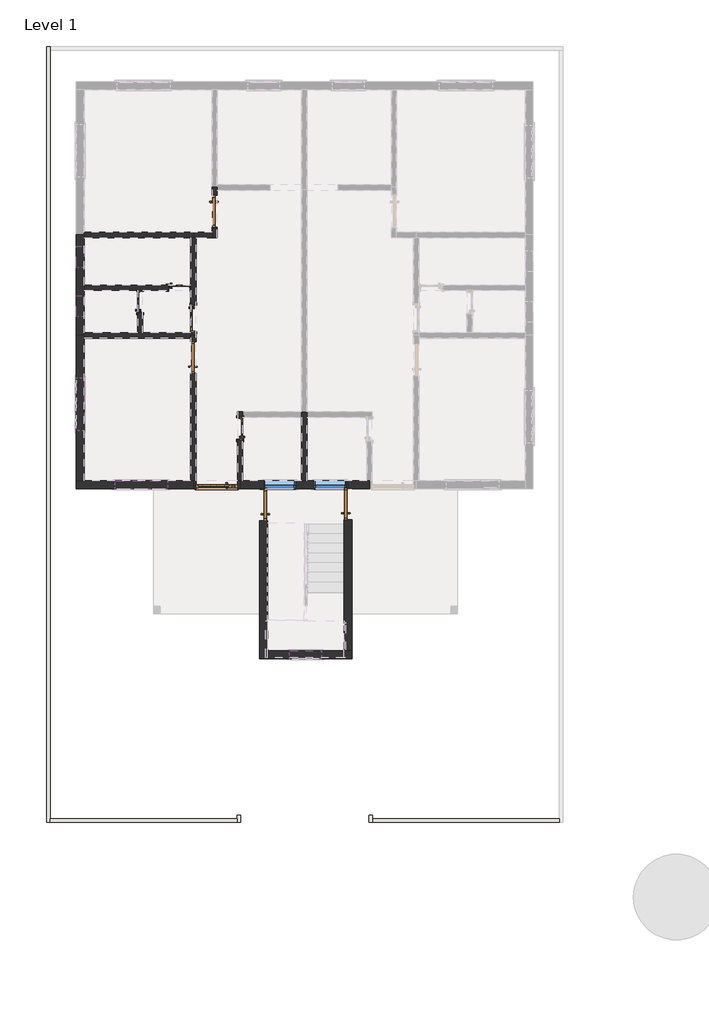
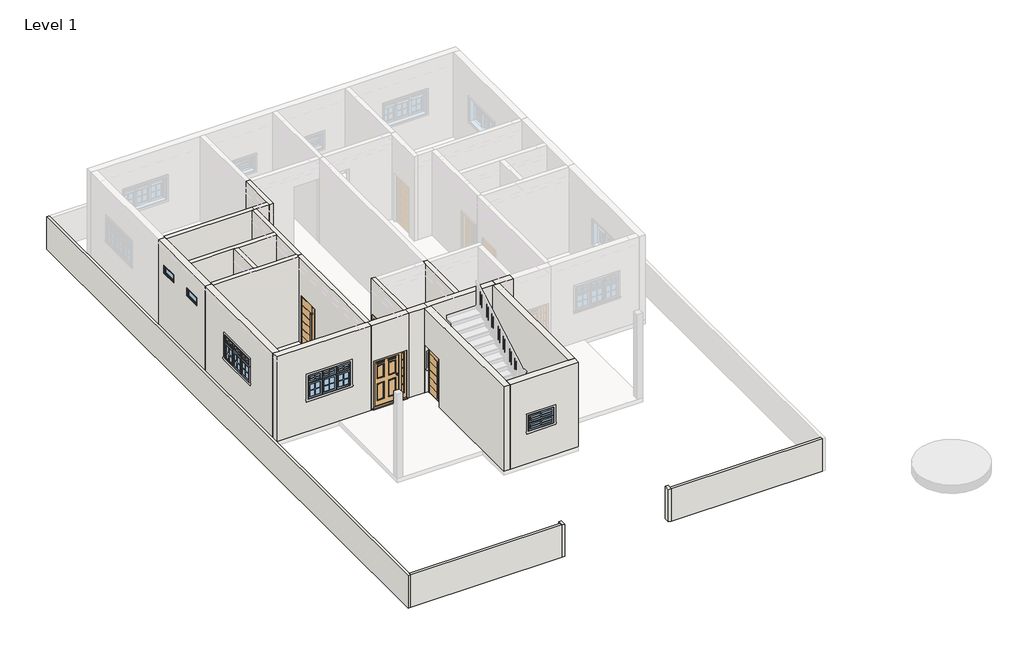
# One storey, part 1 of 4: 25 walls, 9 doors, 7 windows.
# Revit data of these elements (continued)
# Element 38 (IfcWindow, "M_Window-Awning-Double-Vertical : 3'") (continued)
#   Materials on its faces: "Wood - Stained", "Glass", "Clad - White"
# Element 39 (IfcWindow, "M_Window-Awning-Double-Vertical : 3'")
#   Mark = "17"
#   Window Inset = 0' - 0"
#   Interior Wall Closure = 0' - 2.15551"
#   Frame Extension = 0' - 0 1/4"
#   Exterior Wall Closure = 0' - 1 1/4"
#   Interior Trim Visibility = yes
#   Exterior Trim Visibility = yes
#   Phase Created = New Construction
#   Materials on its faces: "Wood - Stained", "Glass", "Clad - White"
# Element 40 (IfcWindow, "M_Window-Casement-Triple-Awning-Triple : 5'")
#   Mark = "7"
#   Window Inset = 0' - 0"
#   Interior Wall Closure = 0' - 2.15551"
#   Frame Extension = 0' - 0 1/4"
#   Exterior Wall Closure = 0' - 1 1/4"
#   Interior Trim Visibility = yes
#   Exterior Trim Visibility = yes
#   Phase Created = New Construction
#   Materials on its faces: "Wood - Stained", "Glass", "Clad - White"
# Element 41 (IfcWindow, "M_Window-Casement-Triple-Awning-Triple : 5'")
#   Mark = "8"
#   Window Inset = 0' - 0"
#   Interior Wall Closure = 0' - 2.15551"
#   Frame Extension = 0' - 0 1/4"
#   Exterior Wall Closure = 0' - 1 1/4"
#   Interior Trim Visibility = yes
#   Exterior Trim Visibility = yes
#   Phase Created = New Construction
#   Materials on its faces: "Wood - Stained", "Glass", "Clad - White"
# Materials
#   "Door - Glazing": colour RGB 0 0 255, transparency 0.75
#   "Door - Panel": class "Wood", colour RGB 210 159 95, transparency 0, Cost = 0
#   "Door - Handle": colour RGB 246 240 166, transparency 0
#   "Cherry": class "Wood", colour RGB 226 177 128, transparency 0, Description = "Prunus Serotina", Cost = 0
#   "Aluminum": class "Metal", colour RGB 247 247 247, transparency 0, Description = "Aluminum 6061", Cost = 0
#   "Glass": class "Glass", colour RGB 0 128 192, transparency 0.75, Description = "Soda Lime Glass", Cost = 0
#   "Sash": class "Wood", colour RGB 224 178 126, transparency 0, Cost = 0
#   "Wood - Stained": class "Wood", colour RGB 224 178 126, transparency 0, Cost = 0
#   "Clad - White": class "Wood", colour RGB 242 242 238, transparency 0, Cost = 0
#   "LVW1": class "Generic", colour RGB 120 120 120, transparency 0, Cost = 0
#   "Default Wall": colour RGB 128 128 128, transparency 0, Cost = 0
#   "BED ROOM WALL 2": class "Generic", colour RGB 120 120 120, transparency 0, Cost = 0
#   "BAW1": class "Generic", colour RGB 120 120 120, transparency 0, Cost = 0
#   "BAW2": class "Generic", colour RGB 120 120 120, transparency 0, Cost = 0
#   "BED ROOM WALL 1": class "Generic", colour RGB 120 120 120, transparency 0, Cost = 0
